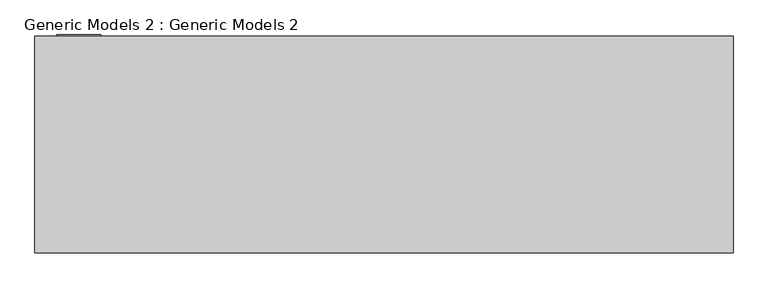
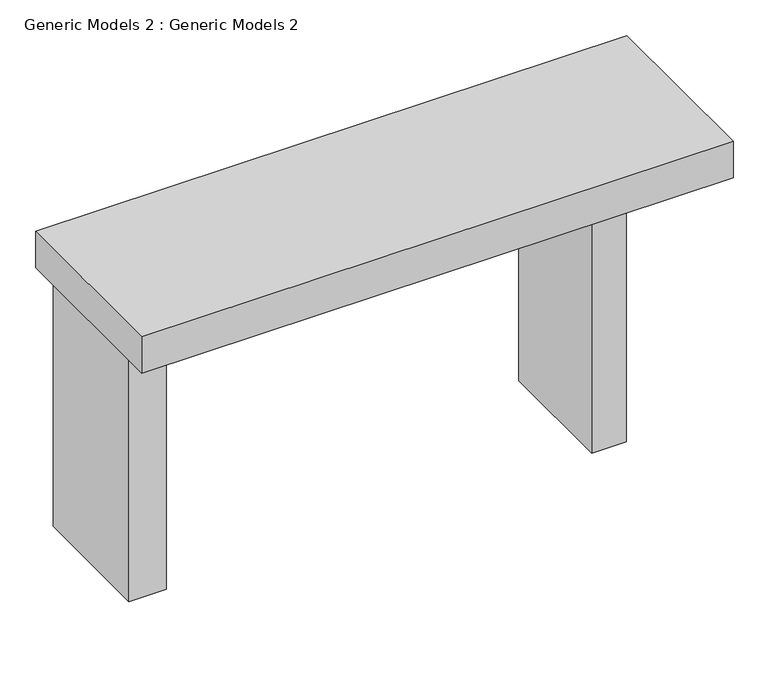
"""IFC4 building model written with IfcOpenShell, lengths in millimetres: proxy geometry, Generic Models 2 : Generic Models 2."""

from ifc_helpers import new_model, si_unit, frame, origin, origin_with_axes, place, context, project, spatial, polyline, outline, extrude, source, transform, mapped, element, save


def generic_models_2_generic_models_2_6fa839af(model_context):
    return source(origin(), model_context, "Body", "SweptSolid", [
        extrude(outline(polyline([(-13736.7607506, -15621.1149487), (-19384.5434854, -15621.1149487), (-19384.5434854, -13864.3466243), (-13736.7607506, -13864.3466243), (-13736.7607506, -15621.1149487)])), frame((0.0, 0.0, 2678.7342332), z_axis=(0.0, 0.0, 1.0), x_axis=(1.0, 0.0, 0.0)), (0.0, 0.0, 1.0), 369.2657668),
        extrude(outline(polyline([(-14456.9434854, -13895.5094868), (-14456.9434854, -15103.8931134), (-14788.414323, -15103.8931134), (-14788.414323, -13895.5094868), (-14456.9434854, -13895.5094868)])), frame((0.0, 0.0, -50.8), z_axis=(0.0, 0.0, 1.0), x_axis=(1.0, 0.0, 0.0)), (0.0, 0.0, 1.0), 2729.5342332),
        extrude(outline(polyline([(-19208.014323, -15103.8931134), (-19208.014323, -13854.1538163), (-18852.414323, -13854.1538163), (-18852.414323, -15103.8931134), (-19208.014323, -15103.8931134)])), origin_with_axes(), (0.0, 0.0, 1.0), 2678.7342332),
    ])


if __name__ == "__main__":
    model = new_model("IFC4")
    model_context = context("Model", 3, world=origin())
    ifc_project = project(units=[si_unit("LENGTHUNIT", "METRE", prefix="MILLI")], contexts=[model_context])
    site = spatial("IfcSite", under=ifc_project)
    building = spatial("IfcBuilding", under=site)
    placement = place(None, origin())
    generic_models_2_generic_models_2_shape = generic_models_2_generic_models_2_6fa839af(model_context)
    element("IfcBuildingElementProxy", 1, Name="Generic Models 2 : Generic Models 2", ObjectType="Generic Models 2 : Generic Models 2", at=placement, inside=building, context=model_context, shape_type="MappedRepresentation", body=[
        mapped(generic_models_2_generic_models_2_shape, transform((0.0, 0.0, 0.0), x_axis=(1.0, 0.0, 0.0), y_axis=(0.0, 1.0, 0.0), z_axis=(0.0, 0.0, 1.0))),
    ])
    save(model, "model.ifc")
